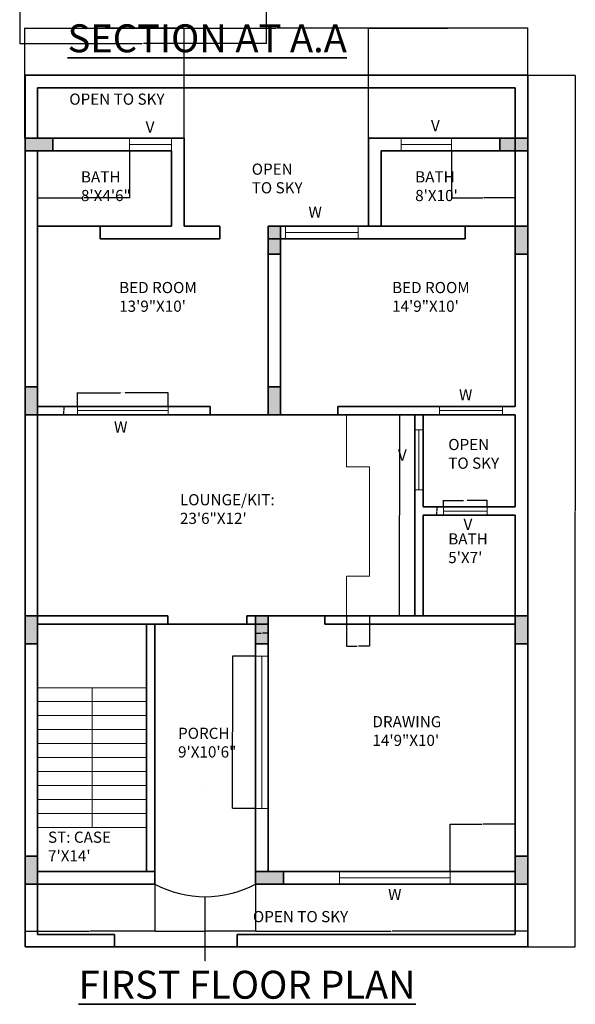
# Model space of a CAD drawing. Units: inches. Extents: x -29 to 834, y -635 to 572.
# Tile 2 of 4: x 434 to 832, y -635 to 69. Entities that reach past the tile are written whole.
import ezdxf

# ---------------------------------------------------------------- set-up
doc = ezdxf.new("R2010")
doc.units = ezdxf.units.IN
doc.header["$MEASUREMENT"] = 0
for name, color, linetype, lineweight in [('A-ANNO-DIMS', 2, 'Continuous', 18), ('A-ANNO-TITL', 7, 'Continuous', 35), ('A-AREA-IDEN', 7, 'Continuous', 18), ('A-COLS', 7, 'Continuous', 35), ('A-FLOR', 7, 'Continuous', 25), ('A-FLOR-FIXT', 8, 'Continuous', 18), ('A-FLOR-STRS', 3, 'Continuous', 18), ('A-GLAZ', 4, 'Continuous', 18), ('A-GLAZ-IDEN', 3, 'Continuous', 18), ('A-WALL', 7, 'Continuous', 35), ('C-PROP', 7, 'Continuous', 35)]:
    doc.layers.add(name, color=color, linetype=linetype, lineweight=lineweight)
doc.styles.get("Standard").update_dxf_attribs({"font": 'arial.ttf'})
doc.dimstyles.get("Standard").update_dxf_attribs({"dimtxt": 0.18, "dimasz": 0.18, "dimexe": 0.18, "dimexo": 0.0625, "dimgap": 0.09, "dimtad": 0, "dimtih": 1, "dimtoh": 1, "dimdec": 4, "dimzin": 0, "dimdsep": 46, "dimtxsty": 'Standard', "dimcen": 0.09, "dimadec": 0, "dimazin": 0, "dimtfac": 1, "dimtdec": 4, "dimtofl": 0, "dimtmove": 0, "dimatfit": 3, "dimfxl": 1, "dimtolj": 1, "dimtzin": 0, "dimarcsym": 0})

# ---------------------------------------------------------------- blocks, each defined once
blk = doc.blocks.new('STAIR-PLAN-RETURN-FLIGHT')
for p, q in [((78, 100), (0, 100)), ((39, 100), (39, 0)), ((78, 90), (0, 90)), ((78, 80), (0, 80)), ((78, 70), (0, 70)), ((78, 60), (0, 60)), ((78, 50), (0, 50)), ((78, 40), (0, 40)), ((78, 30), (0, 30)), ((78, 20), (0, 20)), ((78, 10), (0, 10)), ((78, 0), (0, 0))]:
    blk.add_line(p, q)
blk = doc.blocks.new('KITCHEN-COUNTER-PLAN')
for p, q in [((0, 144), (0, 106.7)), ((0, 106.7), (16.48, 106.7)), ((16.48, 106.7), (16.48, 28.5)), ((16.48, 28.5), (0, 28.5)), ((0, 28.5), (0, 0))]:
    blk.add_line(p, q)
blk = doc.blocks.new('WIN-DRAWING-FRONT-PLAN')
for p, q in [((0, 9), (0, 0)), ((79.05, 9), (79.05, 0)), ((79.05, 4.5), (0, 4.5))]:
    blk.add_line(p, q)
blk = doc.blocks.new('WIN-PORCH-SIDE-PLAN')
for p, q in [((9, 109.08), (0, 109.08)), ((4.5, 0), (4.5, 109.08)), ((9, 0), (0, 0))]:
    blk.add_line(p, q)
blk = doc.blocks.new('WIN-BEDROOM-LOUNGE-PLAN')
for p, q in [((0, 0), (0, 6)), ((64.98, 3), (0, 3)), ((64.98, 0), (64.98, 6))]:
    blk.add_line(p, q)
blk = doc.blocks.new('VENT-LIGHTWELL-SIDE-PLAN')
for p, q in [((6, 43.01), (0, 43.01)), ((3, 0), (3, 43.01)), ((6, 0), (0, 0))]:
    blk.add_line(p, q)
blk = doc.blocks.new('WIN-BEDROOM-REAR-PLAN')
for p, q in [((0, 9), (0, 0)), ((52.22, 9), (52.22, 0)), ((0, 4.5), (52.22, 4.5))]:
    blk.add_line(p, q)
blk = doc.blocks.new('VENT-BATH-LIGHTWELL-PLAN')
for p, q in [((0, 0), (0, 6)), ((31.44, 3), (0, 3)), ((31.44, 0), (31.44, 6))]:
    blk.add_line(p, q)
blk = doc.blocks.new('WIN-BEDROOM-LIGHTWELL-PLAN')
for p, q in [((0, 6), (0, 0)), ((0, 3), (45.04, 3)), ((45.04, 6), (45.04, 0))]:
    blk.add_line(p, q)
blk = doc.blocks.new('VENT-REAR-BATH-R-PLAN')
for p, q in [((0, 9), (0, 0)), ((35.81, 9), (35.81, 0)), ((0, 4.5), (35.81, 4.5))]:
    blk.add_line(p, q)
blk = doc.blocks.new('VENT-REAR-BATH-L-PLAN')
for p, q in [((0, 9), (0, 0)), ((30.05, 9), (30.05, 0)), ((0, 4.5), (30.05, 4.5))]:
    blk.add_line(p, q)
blk = doc.blocks.new('COLUMN-9X20-PLAN')
h = blk.add_hatch(color=256)
h.dxf.hatch_style = 1
h.paths.add_polyline_path([(9, 20), (0, 20), (0, 0), (9, 0)])
blk.add_lwpolyline([(0, 20), (9, 20), (9, 0), (0, 0)], close=True)
blk = doc.blocks.new('*D25')
at = {"layer": 'A-ANNO-DIMS', "color": 0, "lineweight": -2, "transparency": 16777216}
for p, q in [((684.21, -213.46), (705.92, -213.46)), ((705.74, -213.64), (705.74, -285.27)), ((705.74, -357.28), (705.74, -285.64)), ((684.21, -357.46), (705.92, -357.46))]:
    blk.add_line(p, q, dxfattribs=at)
at = {"layer": 'A-ANNO-DIMS', "color": 0, "transparency": 16777216}
for points in [[(705.71, -213.64), (705.77, -213.64), (705.74, -213.46)], [(705.71, -357.28), (705.77, -357.28), (705.74, -357.46)]]:
    blk.add_solid(points, dxfattribs=at)
at = {"layer": 'DEFPOINTS', "color": 0, "transparency": 16777216}
for p in [(684.14, -213.46), (705.74, -213.46), (684.14, -357.46)]:
    blk.add_point(p, dxfattribs=at)
at = {"layer": 'A-ANNO-DIMS', "color": 0, "transparency": 16777216, "insert": (705.74, -285.46), "char_height": 0.18, "attachment_point": 5}
blk.add_mtext('\\A1;COUNTER 144 TYP.', dxfattribs=at)
blk = doc.blocks.new('*D26')
at = {"layer": 'A-ANNO-DIMS', "color": 0, "lineweight": -2, "transparency": 16777216}
for p, q in [((667.66, -357.52), (667.66, -379.24)), ((684.14, -357.52), (684.14, -379.24)), ((667.84, -379.06), (675.38, -379.06)), ((683.96, -379.06), (676.42, -379.06))]:
    blk.add_line(p, q, dxfattribs=at)
at = {"layer": 'A-ANNO-DIMS', "color": 0, "transparency": 16777216}
for points in [[(667.84, -379.03), (667.84, -379.09), (667.66, -379.06)], [(683.96, -379.03), (683.96, -379.09), (684.14, -379.06)]]:
    blk.add_solid(points, dxfattribs=at)
at = {"layer": 'DEFPOINTS', "color": 0, "transparency": 16777216}
for p in [(667.66, -357.46), (684.14, -357.46), (684.14, -379.06)]:
    blk.add_point(p, dxfattribs=at)
at = {"layer": 'A-ANNO-DIMS', "color": 0, "transparency": 16777216, "insert": (675.9, -379.06), "char_height": 0.18, "attachment_point": 5}
blk.add_mtext('\\A1;16 TYP.', dxfattribs=at)
blk = doc.blocks.new('*D29')
at = {"layer": 'A-ANNO-DIMS', "color": 0, "lineweight": -2, "transparency": 16777216}
for p, q in [((602.5, -386.17), (586.02, -386.17)), ((586.2, -386.35), (586.2, -440.52)), ((586.2, -495.06), (586.2, -440.89)), ((602.5, -495.24), (586.02, -495.24))]:
    blk.add_line(p, q, dxfattribs=at)
at = {"layer": 'A-ANNO-DIMS', "color": 0, "transparency": 16777216}
for points in [[(586.17, -386.35), (586.23, -386.35), (586.2, -386.17)], [(586.17, -495.06), (586.23, -495.06), (586.2, -495.24)]]:
    blk.add_solid(points, dxfattribs=at)
at = {"layer": 'DEFPOINTS', "color": 0, "transparency": 16777216}
for p in [(602.56, -386.17), (586.2, -495.24), (602.56, -495.24)]:
    blk.add_point(p, dxfattribs=at)
at = {"layer": 'A-ANNO-DIMS', "color": 0, "transparency": 16777216, "insert": (586.2, -440.71), "char_height": 0.18, "attachment_point": 5}
blk.add_mtext('\\A1;PORCH WINDOW 109 TYP.', dxfattribs=at)
blk = doc.blocks.new('*D30')
at = {"layer": 'A-ANNO-DIMS', "color": 0, "lineweight": -2, "transparency": 16777216}
for p, q in [((602.56, -386.1), (602.56, -369.62)), ((602.74, -369.8), (606.6, -369.8)), ((611.38, -369.8), (607.52, -369.8)), ((611.56, -386.1), (611.56, -369.62))]:
    blk.add_line(p, q, dxfattribs=at)
at = {"layer": 'A-ANNO-DIMS', "color": 0, "transparency": 16777216}
for points in [[(602.74, -369.77), (602.74, -369.83), (602.56, -369.8)], [(611.38, -369.77), (611.38, -369.83), (611.56, -369.8)]]:
    blk.add_solid(points, dxfattribs=at)
at = {"layer": 'DEFPOINTS', "color": 0, "transparency": 16777216}
for p in [(602.56, -369.8), (602.56, -386.17), (611.56, -386.17)]:
    blk.add_point(p, dxfattribs=at)
at = {"layer": 'A-ANNO-DIMS', "color": 0, "transparency": 16777216, "insert": (607.06, -369.8), "char_height": 0.18, "attachment_point": 5}
blk.add_mtext('\\A1;9 TYP.', dxfattribs=at)
blk = doc.blocks.new('*D31')
at = {"layer": 'A-ANNO-DIMS', "color": 0, "lineweight": -2, "transparency": 16777216}
for p, q in [((475.12, -207.39), (475.12, -197.53)), ((475.3, -197.71), (505.93, -197.71)), ((539.92, -197.71), (509.29, -197.71)), ((540.1, -207.39), (540.1, -197.53))]:
    blk.add_line(p, q, dxfattribs=at)
at = {"layer": 'A-ANNO-DIMS', "color": 0, "transparency": 16777216}
for points in [[(475.3, -197.68), (475.3, -197.74), (475.12, -197.71)], [(539.92, -197.68), (539.92, -197.74), (540.1, -197.71)]]:
    blk.add_solid(points, dxfattribs=at)
at = {"layer": 'DEFPOINTS', "color": 0, "transparency": 16777216}
for p in [(475.12, -197.71), (475.12, -207.46), (540.1, -207.46)]:
    blk.add_point(p, dxfattribs=at)
at = {"layer": 'A-ANNO-DIMS', "color": 0, "transparency": 16777216, "insert": (507.61, -197.71), "char_height": 0.18, "attachment_point": 5}
blk.add_mtext('\\A1;LOUNGE WINDOW 65 TYP.', dxfattribs=at)
blk = doc.blocks.new('*D32')
at = {"layer": 'A-ANNO-DIMS', "color": 0, "lineweight": -2, "transparency": 16777216}
for p, q in [((475.06, -207.46), (465.2, -207.46)), ((465.38, -207.64), (465.38, -210.28)), ((465.38, -213.28), (465.38, -210.64)), ((475.06, -213.46), (465.2, -213.46))]:
    blk.add_line(p, q, dxfattribs=at)
at = {"layer": 'A-ANNO-DIMS', "color": 0, "transparency": 16777216}
for points in [[(465.35, -207.64), (465.41, -207.64), (465.38, -207.46)], [(465.35, -213.28), (465.41, -213.28), (465.38, -213.46)]]:
    blk.add_solid(points, dxfattribs=at)
at = {"layer": 'DEFPOINTS', "color": 0, "transparency": 16777216}
for p in [(475.12, -207.46), (465.38, -213.46), (475.12, -213.46)]:
    blk.add_point(p, dxfattribs=at)
at = {"layer": 'A-ANNO-DIMS', "color": 0, "transparency": 16777216, "insert": (465.38, -210.46), "char_height": 0.18, "attachment_point": 5}
blk.add_mtext('\\A1;6 TYP.', dxfattribs=at)
blk = doc.blocks.new('*D37')
at = {"layer": 'A-ANNO-DIMS', "color": 0, "lineweight": -2, "transparency": 16777216}
for p, q in [((737.12, -279.39), (737.12, -274.56)), ((737.3, -274.74), (751.58, -274.74)), ((768.38, -274.74), (754.1, -274.74)), ((768.56, -279.39), (768.56, -274.56))]:
    blk.add_line(p, q, dxfattribs=at)
at = {"layer": 'A-ANNO-DIMS', "color": 0, "transparency": 16777216}
for points in [[(737.3, -274.71), (737.3, -274.77), (737.12, -274.74)], [(768.38, -274.71), (768.38, -274.77), (768.56, -274.74)]]:
    blk.add_solid(points, dxfattribs=at)
at = {"layer": 'DEFPOINTS', "color": 0, "transparency": 16777216}
for p in [(737.12, -274.74), (737.12, -279.46), (768.56, -279.46)]:
    blk.add_point(p, dxfattribs=at)
at = {"layer": 'A-ANNO-DIMS', "color": 0, "transparency": 16777216, "insert": (752.84, -274.74), "char_height": 0.18, "attachment_point": 5}
blk.add_mtext('\\A1;BATH VENT 31 TYP.', dxfattribs=at)
blk = doc.blocks.new('*D38')
at = {"layer": 'A-ANNO-DIMS', "color": 0, "lineweight": -2, "transparency": 16777216}
for p, q in [((737.06, -279.46), (732.22, -279.46)), ((732.4, -279.64), (732.4, -282.28)), ((737.06, -285.46), (732.22, -285.46)), ((732.4, -285.28), (732.4, -282.64))]:
    blk.add_line(p, q, dxfattribs=at)
at = {"layer": 'A-ANNO-DIMS', "color": 0, "transparency": 16777216}
for points in [[(732.37, -279.64), (732.43, -279.64), (732.4, -279.46)], [(732.37, -285.28), (732.43, -285.28), (732.4, -285.46)]]:
    blk.add_solid(points, dxfattribs=at)
at = {"layer": 'DEFPOINTS', "color": 0, "transparency": 16777216}
for p in [(737.12, -279.46), (732.4, -285.46), (737.12, -285.46)]:
    blk.add_point(p, dxfattribs=at)
at = {"layer": 'A-ANNO-DIMS', "color": 0, "transparency": 16777216, "insert": (732.4, -282.46), "char_height": 0.18, "attachment_point": 5}
blk.add_mtext('\\A1;6 TYP.', dxfattribs=at)
blk = doc.blocks.new('*D61')
at = {"layer": 'A-ANNO-DIMS', "color": 0, "lineweight": -2, "transparency": 16777216}
for p, q in [((437.56, 29.61), (437.56, 63.52)), ((797.56, 29.61), (797.56, 63.52)), ((437.74, 63.34), (617.27, 63.34)), ((797.38, 63.34), (617.85, 63.34))]:
    blk.add_line(p, q, dxfattribs=at)
at = {"layer": 'A-ANNO-DIMS', "color": 0, "transparency": 16777216}
for points in [[(437.74, 63.37), (437.74, 63.31), (437.56, 63.34)], [(797.38, 63.37), (797.38, 63.31), (797.56, 63.34)]]:
    blk.add_solid(points, dxfattribs=at)
at = {"layer": 'DEFPOINTS', "color": 0, "transparency": 16777216}
for p in [(797.56, 63.34), (437.56, 29.54), (797.56, 29.54)]:
    blk.add_point(p, dxfattribs=at)
at = {"layer": 'A-ANNO-DIMS', "color": 0, "transparency": 16777216, "insert": (617.56, 63.34), "char_height": 0.18, "attachment_point": 5}
blk.add_mtext('\\A1;360', dxfattribs=at)
blk = doc.blocks.new('*D62')
at = {"layer": 'A-ANNO-DIMS', "color": 0, "lineweight": -2, "transparency": 16777216}
for p, q in [((797.63, 29.54), (831.54, 29.54)), ((831.36, 29.36), (831.36, -282.28)), ((831.36, -594.28), (831.36, -282.64)), ((797.63, -594.46), (831.54, -594.46))]:
    blk.add_line(p, q, dxfattribs=at)
at = {"layer": 'A-ANNO-DIMS', "color": 0, "transparency": 16777216}
for points in [[(831.33, 29.36), (831.39, 29.36), (831.36, 29.54)], [(831.33, -594.28), (831.39, -594.28), (831.36, -594.46)]]:
    blk.add_solid(points, dxfattribs=at)
at = {"layer": 'DEFPOINTS', "color": 0, "transparency": 16777216}
for p in [(797.56, 29.54), (831.36, 29.54), (797.56, -594.46)]:
    blk.add_point(p, dxfattribs=at)
at = {"layer": 'A-ANNO-DIMS', "color": 0, "transparency": 16777216, "insert": (831.36, -282.46), "char_height": 0.18, "attachment_point": 5}
blk.add_mtext('\\A1;624', dxfattribs=at)
blk = doc.blocks.new('*D63')
at = {"layer": 'A-ANNO-DIMS', "color": 0, "lineweight": -2, "transparency": 16777216}
for p, q in [((437.56, -549.52), (437.56, -583.44)), ((530.56, -549.52), (530.56, -583.44)), ((437.74, -583.26), (483.84, -583.26)), ((530.38, -583.26), (484.28, -583.26))]:
    blk.add_line(p, q, dxfattribs=at)
at = {"layer": 'A-ANNO-DIMS', "color": 0, "transparency": 16777216}
for points in [[(437.74, -583.23), (437.74, -583.29), (437.56, -583.26)], [(530.38, -583.23), (530.38, -583.29), (530.56, -583.26)]]:
    blk.add_solid(points, dxfattribs=at)
at = {"layer": 'DEFPOINTS', "color": 0, "transparency": 16777216}
for p in [(437.56, -549.46), (530.56, -549.46), (437.56, -583.26)]:
    blk.add_point(p, dxfattribs=at)
at = {"layer": 'A-ANNO-DIMS', "color": 0, "transparency": 16777216, "insert": (484.06, -583.26), "char_height": 0.18, "attachment_point": 5}
blk.add_mtext('\\A1;93', dxfattribs=at)
blk = doc.blocks.new('*D64')
at = {"layer": 'A-ANNO-DIMS', "color": 0, "lineweight": -2, "transparency": 16777216}
for p, q in [((530.56, -549.52), (530.56, -583.44)), ((602.56, -549.52), (602.56, -583.44)), ((530.74, -583.26), (566.35, -583.26)), ((602.38, -583.26), (566.78, -583.26))]:
    blk.add_line(p, q, dxfattribs=at)
at = {"layer": 'A-ANNO-DIMS', "color": 0, "transparency": 16777216}
for points in [[(530.74, -583.23), (530.74, -583.29), (530.56, -583.26)], [(602.38, -583.23), (602.38, -583.29), (602.56, -583.26)]]:
    blk.add_solid(points, dxfattribs=at)
at = {"layer": 'DEFPOINTS', "color": 0, "transparency": 16777216}
for p in [(530.56, -549.46), (602.56, -549.46), (530.56, -583.26)]:
    blk.add_point(p, dxfattribs=at)
at = {"layer": 'A-ANNO-DIMS', "color": 0, "transparency": 16777216, "insert": (566.56, -583.26), "char_height": 0.18, "attachment_point": 5}
blk.add_mtext('\\A1;72', dxfattribs=at)
blk = doc.blocks.new('*D65')
at = {"layer": 'A-ANNO-DIMS', "color": 0, "lineweight": -2, "transparency": 16777216}
for p, q in [((602.56, -549.52), (602.56, -583.44)), ((797.56, -549.52), (797.56, -583.44)), ((602.74, -583.26), (699.78, -583.26)), ((797.38, -583.26), (700.34, -583.26))]:
    blk.add_line(p, q, dxfattribs=at)
at = {"layer": 'A-ANNO-DIMS', "color": 0, "transparency": 16777216}
for points in [[(602.74, -583.23), (602.74, -583.29), (602.56, -583.26)], [(797.38, -583.23), (797.38, -583.29), (797.56, -583.26)]]:
    blk.add_solid(points, dxfattribs=at)
at = {"layer": 'DEFPOINTS', "color": 0, "transparency": 16777216}
for p in [(602.56, -549.46), (797.56, -549.46), (602.56, -583.26)]:
    blk.add_point(p, dxfattribs=at)
at = {"layer": 'A-ANNO-DIMS', "color": 0, "transparency": 16777216, "insert": (700.06, -583.26), "char_height": 0.18, "attachment_point": 5}
blk.add_mtext('\\A1;195', dxfattribs=at)
blk = doc.blocks.new('*D72')
at = {"layer": 'A-ANNO-DIMS', "color": 0, "lineweight": -2, "transparency": 16777216}
for p, q in [((437.56, -15.39), (437.56, 63.52)), ((551.56, -15.39), (551.56, 63.52)), ((437.74, 63.34), (494.28, 63.34)), ((551.38, 63.34), (494.84, 63.34))]:
    blk.add_line(p, q, dxfattribs=at)
at = {"layer": 'A-ANNO-DIMS', "color": 0, "transparency": 16777216}
for points in [[(437.74, 63.37), (437.74, 63.31), (437.56, 63.34)], [(551.38, 63.37), (551.38, 63.31), (551.56, 63.34)]]:
    blk.add_solid(points, dxfattribs=at)
at = {"layer": 'DEFPOINTS', "color": 0, "transparency": 16777216}
for p in [(551.56, 63.34), (437.56, -15.46), (551.56, -15.46)]:
    blk.add_point(p, dxfattribs=at)
at = {"layer": 'A-ANNO-DIMS', "color": 0, "transparency": 16777216, "insert": (494.56, 63.34), "char_height": 0.18, "attachment_point": 5}
blk.add_mtext('\\A1;114', dxfattribs=at)
blk = doc.blocks.new('*D73')
at = {"layer": 'A-ANNO-DIMS', "color": 0, "lineweight": -2, "transparency": 16777216}
for p, q in [((551.56, -15.39), (551.56, 63.52)), ((683.56, -15.39), (683.56, 63.52)), ((551.74, 63.34), (617.28, 63.34)), ((683.38, 63.34), (617.84, 63.34))]:
    blk.add_line(p, q, dxfattribs=at)
at = {"layer": 'A-ANNO-DIMS', "color": 0, "transparency": 16777216}
for points in [[(551.74, 63.37), (551.74, 63.31), (551.56, 63.34)], [(683.38, 63.37), (683.38, 63.31), (683.56, 63.34)]]:
    blk.add_solid(points, dxfattribs=at)
at = {"layer": 'DEFPOINTS', "color": 0, "transparency": 16777216}
for p in [(683.56, 63.34), (551.56, -15.46), (683.56, -15.46)]:
    blk.add_point(p, dxfattribs=at)
at = {"layer": 'A-ANNO-DIMS', "color": 0, "transparency": 16777216, "insert": (617.56, 63.34), "char_height": 0.18, "attachment_point": 5}
blk.add_mtext('\\A1;132', dxfattribs=at)
blk = doc.blocks.new('*D74')
at = {"layer": 'A-ANNO-DIMS', "color": 0, "lineweight": -2, "transparency": 16777216}
for p, q in [((683.56, -15.39), (683.56, 63.52)), ((797.56, -15.39), (797.56, 63.52)), ((683.74, 63.34), (740.28, 63.34)), ((797.38, 63.34), (740.84, 63.34))]:
    blk.add_line(p, q, dxfattribs=at)
at = {"layer": 'A-ANNO-DIMS', "color": 0, "transparency": 16777216}
for points in [[(683.74, 63.37), (683.74, 63.31), (683.56, 63.34)], [(797.38, 63.37), (797.38, 63.31), (797.56, 63.34)]]:
    blk.add_solid(points, dxfattribs=at)
at = {"layer": 'DEFPOINTS', "color": 0, "transparency": 16777216}
for p in [(797.56, 63.34), (683.56, -15.46), (797.56, -15.46)]:
    blk.add_point(p, dxfattribs=at)
at = {"layer": 'A-ANNO-DIMS', "color": 0, "transparency": 16777216, "insert": (740.56, 63.34), "char_height": 0.18, "attachment_point": 5}
blk.add_mtext('\\A1;114', dxfattribs=at)
blk = doc.blocks.new('*D75')
at = {"layer": 'A-ANNO-DIMS', "color": 0, "lineweight": -2, "transparency": 16777216}
for p, q in [((446.56, -24.52), (446.56, -58.44)), ((512.45, -24.52), (512.45, -58.44)), ((446.74, -58.26), (479.11, -58.26)), ((512.27, -58.26), (479.9, -58.26))]:
    blk.add_line(p, q, dxfattribs=at)
at = {"layer": 'A-ANNO-DIMS', "color": 0, "transparency": 16777216}
for points in [[(446.74, -58.23), (446.74, -58.29), (446.56, -58.26)], [(512.27, -58.23), (512.27, -58.29), (512.45, -58.26)]]:
    blk.add_solid(points, dxfattribs=at)
at = {"layer": 'DEFPOINTS', "color": 0, "transparency": 16777216}
for p in [(446.56, -24.46), (512.45, -24.46), (446.56, -58.26)]:
    blk.add_point(p, dxfattribs=at)
at = {"layer": 'A-ANNO-DIMS', "color": 0, "transparency": 16777216, "insert": (479.51, -58.26), "char_height": 0.18, "attachment_point": 5}
blk.add_mtext('\\A1;65.89', dxfattribs=at)
blk = doc.blocks.new('*D76')
at = {"layer": 'A-ANNO-DIMS', "color": 0, "lineweight": -2, "transparency": 16777216}
for p, q in [((742.81, -24.52), (742.81, -58.44)), ((788.56, -24.52), (788.56, -58.44)), ((742.99, -58.26), (765.29, -58.26)), ((788.38, -58.26), (766.08, -58.26))]:
    blk.add_line(p, q, dxfattribs=at)
at = {"layer": 'A-ANNO-DIMS', "color": 0, "transparency": 16777216}
for points in [[(742.99, -58.23), (742.99, -58.29), (742.81, -58.26)], [(788.38, -58.23), (788.38, -58.29), (788.56, -58.26)]]:
    blk.add_solid(points, dxfattribs=at)
at = {"layer": 'DEFPOINTS', "color": 0, "transparency": 16777216}
for p in [(742.81, -24.46), (788.56, -24.46), (742.81, -58.26)]:
    blk.add_point(p, dxfattribs=at)
at = {"layer": 'A-ANNO-DIMS', "color": 0, "transparency": 16777216, "insert": (765.68, -58.26), "char_height": 0.18, "attachment_point": 5}
blk.add_mtext('\\A1;45.76', dxfattribs=at)
blk = doc.blocks.new('*D79')
at = {"layer": 'A-ANNO-DIMS', "color": 0, "lineweight": -2, "transparency": 16777216}
for p, q in [((741.86, -540.39), (741.86, -506.48)), ((742.04, -506.66), (764.88, -506.66)), ((788.38, -506.66), (765.54, -506.66)), ((788.56, -540.39), (788.56, -506.48))]:
    blk.add_line(p, q, dxfattribs=at)
at = {"layer": 'A-ANNO-DIMS', "color": 0, "transparency": 16777216}
for points in [[(742.04, -506.63), (742.04, -506.69), (741.86, -506.66)], [(788.38, -506.63), (788.38, -506.69), (788.56, -506.66)]]:
    blk.add_solid(points, dxfattribs=at)
at = {"layer": 'DEFPOINTS', "color": 0, "transparency": 16777216}
for p in [(788.56, -506.66), (741.86, -540.46), (788.56, -540.46)]:
    blk.add_point(p, dxfattribs=at)
at = {"layer": 'A-ANNO-DIMS', "color": 0, "transparency": 16777216, "insert": (765.21, -506.66), "char_height": 0.18, "attachment_point": 5}
blk.add_mtext('\\A1;46.7', dxfattribs=at)
blk = doc.blocks.new('*D101')
at = {"layer": 'A-ANNO-DIMS', "color": 0, "lineweight": -2, "transparency": 16777216}
for p, q in [((433.76, 110.48), (433.76, 52.17)), ((610.21, 110.48), (610.21, 52.17)), ((433.94, 52.35), (521.53, 52.35)), ((610.03, 52.35), (522.44, 52.35))]:
    blk.add_line(p, q, dxfattribs=at)
at = {"layer": 'A-ANNO-DIMS', "color": 0, "transparency": 16777216}
for points in [[(433.94, 52.38), (433.94, 52.32), (433.76, 52.35)], [(610.03, 52.38), (610.03, 52.32), (610.21, 52.35)]]:
    blk.add_solid(points, dxfattribs=at)
at = {"layer": 'DEFPOINTS', "color": 0, "transparency": 16777216}
for p in [(433.76, 110.54), (610.21, 110.54), (610.21, 52.35)]:
    blk.add_point(p, dxfattribs=at)
at = {"layer": 'A-ANNO-DIMS', "color": 0, "transparency": 16777216, "insert": (521.98, 52.35), "char_height": 0.18, "attachment_point": 5}
blk.add_mtext('\\A1;176.45', dxfattribs=at)
blk = doc.blocks.new('*D108')
at = {"layer": 'A-ANNO-DIMS', "color": 0, "lineweight": -2, "transparency": 16777216}
for p, q in [((566.47, -481.96), (566.65, -481.96)), ((566.56, -482.05), (566.56, -481.87)), ((566.56, -604.36), (566.56, -558.64)), ((566.74, -604.36), (566.56, -604.36))]:
    blk.add_line(p, q, dxfattribs=at)
at = {"layer": 'A-ANNO-DIMS', "color": 0, "transparency": 16777216}
blk.add_solid([(566.59, -558.64), (566.53, -558.64), (566.56, -558.46)], dxfattribs=at)
at = {"layer": 'DEFPOINTS', "color": 0, "transparency": 16777216}
for p in [(566.56, -481.96), (566.56, -558.46)]:
    blk.add_point(p, dxfattribs=at)
at = {"layer": 'A-ANNO-DIMS', "color": 0, "transparency": 16777216, "insert": (567.15, -604.36), "char_height": 0.18, "attachment_point": 5}
blk.add_mtext('\\A1;R76.5', dxfattribs=at)

msp = doc.modelspace()

# ---------------------------------------------------------------- linework, layer by layer
at = {"layer": 'A-FLOR'}
msp.add_arc((566.5626, -481.957), 76.5, 241.9275073, 298.0724927, dxfattribs=at)
at = {"layer": 'A-WALL'}
for p, q in [((446.5626, 20.5431), (788.5626, 20.5431)), ((446.5626, 20.5431), (446.5626, -15.4569)), ((788.5626, 20.5431), (788.5626, -78.4569)), ((446.5626, -15.4569), (551.5626, -15.4569)), ((551.5626, -15.4569), (551.5626, -78.4569)), ((683.5626, -15.4569), (788.5626, -15.4569)), ((683.5626, -15.4569), (683.5626, -78.4569)), ((446.5626, -24.4569), (542.5626, -24.4569)), ((446.5626, -24.4569), (446.5626, -78.4569)), ((542.5626, -24.4569), (542.5626, -78.4569)), ((692.5626, -24.4569), (788.5626, -24.4569)), ((692.5626, -24.4569), (692.5626, -78.4569)), ((446.5626, -78.4569), (542.5626, -78.4569)), ((446.5626, -78.4569), (446.5626, -87.4569)), ((491.4048, -78.4569), (491.4048, -87.4569)), ((551.5626, -78.4569), (577.0558, -78.4569)), ((577.0558, -78.4569), (577.0558, -87.4569)), ((611.5626, -78.4569), (788.5626, -78.4569)), ((611.5626, -78.4569), (611.5626, -207.4569)), ((752.6848, -78.4569), (752.6848, -87.4569)), ((788.5626, -78.4569), (788.5626, -87.4569)), ((446.5626, -87.4569), (446.5626, -207.4569)), ((491.4048, -87.4569), (577.0558, -87.4569)), ((611.5626, -87.4569), (752.6848, -87.4569)), ((620.5626, -87.4569), (620.5626, -207.4569)), ((788.5626, -87.4569), (788.5626, -207.4569)), ((446.5626, -207.4569), (570.1065, -207.4569)), ((570.1065, -207.4569), (570.1065, -213.4569)), ((611.5626, -207.4569), (611.5626, -213.4569)), ((620.5626, -207.4569), (620.5626, -213.4569)), ((661.5051, -207.4569), (788.5626, -207.4569)), ((661.5051, -207.4569), (661.5051, -213.4569)), ((446.5626, -213.4569), (788.5626, -213.4569)), ((446.5626, -213.4569), (446.5626, -357.4569)), ((716.5626, -213.4569), (716.5626, -357.4569)), ((722.5626, -213.4569), (722.5626, -279.4569)), ((788.5626, -213.4569), (788.5626, -279.4569)), ((722.5626, -279.4569), (788.5626, -279.4569)), ((722.5626, -285.4569), (788.5626, -285.4569)), ((722.5626, -285.4569), (722.5626, -357.4569)), ((788.5626, -285.4569), (788.5626, -357.4569)), ((446.5626, -357.4569), (539.8795, -357.4569)), ((539.8795, -357.4569), (539.8795, -363.4569)), ((596.4793, -357.4569), (788.5626, -357.4569)), ((596.4793, -357.4569), (596.4793, -363.4569)), ((611.5626, -363.4569), (611.5626, -357.4569)), ((652.1881, -357.4569), (652.1881, -363.4569)), ((446.5626, -363.4569), (611.5626, -363.4569)), ((446.5626, -363.4569), (446.5626, -540.4569)), ((524.5626, -363.4569), (524.5626, -540.4569)), ((530.5626, -363.4569), (530.5626, -549.4569)), ((602.5626, -363.4569), (602.5626, -549.4569)), ((611.5626, -363.4569), (611.5626, -540.4569)), ((652.1881, -363.4569), (788.5626, -363.4569)), ((788.5626, -363.4569), (788.5626, -540.4569)), ((446.5626, -540.4569), (530.5626, -540.4569)), ((602.5626, -540.4569), (788.5626, -540.4569)), ((446.5626, -549.4569), (530.5626, -549.4569)), ((446.5626, -549.4569), (446.5626, -585.4569)), ((602.5626, -549.4569), (788.5626, -549.4569)), ((788.5626, -549.4569), (788.5626, -585.4569)), ((446.5626, -585.4569), (501.5833, -585.4569)), ((501.5833, -585.4569), (501.5833, -594.4569)), ((589.5168, -585.4569), (788.5626, -585.4569)), ((589.5168, -585.4569), (589.5168, -594.4569))]:
    msp.add_line(p, q, dxfattribs=at)
at = {"layer": 'C-PROP'}
for p, q in [((437.5626, 29.5431), (797.5626, 29.5431)), ((437.5626, 29.5431), (437.5626, -594.4569)), ((797.5626, 29.5431), (797.5626, -594.4569)), ((437.5626, -594.4569), (797.5626, -594.4569))]:
    msp.add_line(p, q, dxfattribs=at)

# ---------------------------------------------------------------- block references
at = {"layer": 'A-COLS'}
for p, rotation in [((437.5626, -15.4569), 270.0000000000002), ((777.5626, -15.4569), 270.0000000000002), ((602.5626, -540.4569), 269.9999999999995)]:
    msp.add_blockref('COLUMN-9X20-PLAN', p, dxfattribs=dict(at, rotation=rotation))
for p in [(611.5626, -98.4569), (788.5626, -98.4569), (437.5626, -213.4569), (611.5626, -213.4569), (437.5626, -377.4569), (602.5626, -377.4569), (788.5626, -377.4569), (437.5626, -549.4569), (788.5626, -549.4569)]:
    msp.add_blockref('COLUMN-9X20-PLAN', p, dxfattribs=at)
at = {"layer": 'A-FLOR-FIXT'}
msp.add_blockref('KITCHEN-COUNTER-PLAN', (667.661, -357.4569), dxfattribs=at)
at = {"layer": 'A-FLOR-STRS'}
msp.add_blockref('STAIR-PLAN-RETURN-FLIGHT', (446.5626, -508.8447), dxfattribs=at)
at = {"layer": 'A-GLAZ'}
for name, p in [('VENT-REAR-BATH-L-PLAN', (512.45, -24.4569)), ('VENT-REAR-BATH-R-PLAN', (707.0002, -24.4569)), ('WIN-BEDROOM-REAR-PLAN', (623.9837, -87.4569)), ('WIN-BEDROOM-LIGHTWELL-PLAN', (734.3077, -213.4569)), ('WIN-DRAWING-FRONT-PLAN', (662.8149, -549.4569))]:
    msp.add_blockref(name, p, dxfattribs=at)
at = {"layer": 'A-GLAZ', "rotation": 180}
for name, p in [('WIN-BEDROOM-LOUNGE-PLAN', (540.0997, -207.4569)), ('VENT-LIGHTWELL-SIDE-PLAN', (722.5626, -224.1814)), ('VENT-BATH-LIGHTWELL-PLAN', (768.5589, -279.4569)), ('WIN-PORCH-SIDE-PLAN', (611.5626, -386.1664))]:
    msp.add_blockref(name, p, dxfattribs=at)

# ---------------------------------------------------------------- texts
at = {"layer": 'A-ANNO-TITL', "char_height": 20, "attachment_point": 1}
for s, insert in [('{\\LSECTION AT A.A}', (468.0427, 66.0256)), ('{\\LFIRST FLOOR PLAN}', (475.9632, -611.4996))]:
    msp.add_mtext_dynamic_manual_height_columns(s, width=384.972308, gutter_width=1, heights=[0], dxfattribs=dict(at, insert=insert))
at = {"layer": 'A-AREA-IDEN', "char_height": 8, "attachment_point": 1}
for s, insert in [('OPEN TO SKY', (469.2703, 16.4692)), ('OPEN\\PTO SKY', (599.8903, -33.6457)), ('BATH\\P8\'X4\'6"', (477.6207, -39.1901)), ("BATH\\P8'X10'", (716.9232, -39.1901)), ('BED ROOM\\P13\'9"X10\'', (504.9938, -118.4186)), ('BED ROOM\\P14\'9"X10\'', (700.4035, -118.4186)), ('OPEN\\PTO SKY', (740.5888, -230.7819)), ('LOUNGE/KIT:\\P23\'6"X12\'', (548.5087, -270.2979)), ("BATH\\P5'X7'", (740.5888, -298.3415)), ('DRAWING\\P14\'9"X10\'', (686.3234, -429.2086)), ('PORCH\\P9\'X10\'6"', (547.1385, -437.4896)), ("ST: CASE\\P7'X14'", (454.0475, -511.8774)), ('OPEN TO SKY', (600.7441, -568.7152))]:
    msp.add_mtext_dynamic_manual_height_columns(s, width=92.580232, gutter_width=1, heights=[0], dxfattribs=dict(at, insert=insert))
at = {"layer": 'A-GLAZ-IDEN', "char_height": 8, "attachment_point": 1}
for s, width, insert in [('V', 15.530915, (523.9493, -3.4402)), ('V', 15.530915, (728.2293, -2.5018)), ('W', 92.580232, (640.5145, -64.4301)), ('W', 92.580232, (748.29, -195.1503)), ('W', 92.580232, (501.3218, -218.2872)), ('V', 15.530915, (704.5498, -238.3243)), ('V', 15.530915, (751.5533, -287.9574)), ('W', 92.580232, (697.5275, -552.8615))]:
    msp.add_mtext_dynamic_manual_height_columns(s, width=width, gutter_width=1, heights=[0], dxfattribs=dict(at, insert=insert))

# ---------------------------------------------------------------- dimensions: what is measured, and where the dimension line sits
at = {"layer": 'A-ANNO-DIMS'}
for base, p1, p2, override, picture, middle in [((610.2079, 52.3492), (433.7594, 110.5416), (610.2079, 110.5416), {"dimdec": 2, "dimlfac": 1, "dimrnd": 0, "dimzin": 0, "dimdsep": 46, "dimlunit": 2}, '*D101', (521.9837, 52.3492)), ((797.5626, 63.3431), (437.5626, 29.5431), (797.5626, 29.5431), {"dimdec": 0, "dimlfac": 1, "dimrnd": 0, "dimzin": 0, "dimdsep": 46, "dimlunit": 2}, '*D61', (617.5626, 63.3431)), ((551.5626, 63.3431), (437.5626, -15.4569), (551.5626, -15.4569), {"dimdec": 0, "dimlfac": 1, "dimrnd": 0, "dimzin": 0, "dimdsep": 46, "dimlunit": 2}, '*D72', (494.5626, 63.3431)), ((683.5626, 63.3431), (551.5626, -15.4569), (683.5626, -15.4569), {"dimdec": 0, "dimlfac": 1, "dimrnd": 0, "dimzin": 0, "dimdsep": 46, "dimlunit": 2}, '*D73', (617.5626, 63.3431)), ((797.5626, 63.3431), (683.5626, -15.4569), (797.5626, -15.4569), {"dimdec": 0, "dimlfac": 1, "dimrnd": 0, "dimzin": 0, "dimdsep": 46, "dimlunit": 2}, '*D74', (740.5626, 63.3431))]:
    dim = msp.add_linear_dim(base=base, p1=p1, p2=p2, dimstyle='Standard', override=override, dxfattribs=at)
    dim.commit()
    dim.dimension.update_dxf_attribs({"geometry": picture, "text_midpoint": middle})
for base, p1, p2, angle, override, picture, middle in [((831.3626, 29.5431), (797.5626, -594.4569), (797.5626, 29.5431), 90, {"dimdec": 0, "dimlfac": 1, "dimrnd": 0, "dimzin": 0, "dimdsep": 46, "dimlunit": 2}, '*D62', (831.3626, -282.4569)), ((446.5626, -58.2569), (512.45, -24.4569), (446.5626, -24.4569), 180, {"dimdec": 2, "dimlfac": 1, "dimrnd": 0, "dimzin": 0, "dimdsep": 46, "dimlunit": 2}, '*D75', (479.5063, -58.2569)), ((742.8066, -58.2569), (788.5626, -24.4569), (742.8066, -24.4569), 180, {"dimdec": 2, "dimlfac": 1, "dimrnd": 0, "dimzin": 0, "dimdsep": 46, "dimlunit": 2}, '*D76', (765.6846, -58.2569)), ((788.5626, -506.6569), (741.8605, -540.4569), (788.5626, -540.4569), 0, {"dimdec": 1, "dimlfac": 1, "dimrnd": 0, "dimzin": 0, "dimdsep": 46, "dimlunit": 2}, '*D79', (765.2115, -506.6569)), ((437.5626, -583.2569), (530.5626, -549.4569), (437.5626, -549.4569), 180, {"dimdec": 0, "dimlfac": 1, "dimrnd": 0, "dimzin": 0, "dimdsep": 46, "dimlunit": 2}, '*D63', (484.0626, -583.2569)), ((530.5626, -583.2569), (602.5626, -549.4569), (530.5626, -549.4569), 180, {"dimdec": 0, "dimlfac": 1, "dimrnd": 0, "dimzin": 0, "dimdsep": 46, "dimlunit": 2}, '*D64', (566.5626, -583.2569)), ((602.5626, -583.2569), (797.5626, -549.4569), (602.5626, -549.4569), 180, {"dimdec": 0, "dimlfac": 1, "dimrnd": 0, "dimzin": 0, "dimdsep": 46, "dimlunit": 2}, '*D65', (700.0626, -583.2569))]:
    dim = msp.add_linear_dim(base=base, p1=p1, p2=p2, angle=angle, dimstyle='Standard', override=override, dxfattribs=at)
    dim.commit()
    dim.dimension.update_dxf_attribs({"geometry": picture, "text_midpoint": middle})
for base, p1, p2, angle, text, picture, middle in [((475.1233, -197.7105), (540.0997, -207.4569), (475.1233, -207.4569), 180, 'LOUNGE WINDOW <> TYP.', '*D31', (507.6115, -197.7105)), ((465.3768, -213.4569), (475.1233, -207.4569), (475.1233, -213.4569), 270, '<> TYP.', '*D32', (465.3768, -210.4569)), ((705.7437, -213.4569), (684.1437, -357.4569), (684.1437, -213.4569), 90, 'COUNTER <> TYP.', '*D25', (705.7437, -285.4569)), ((737.1205, -274.7412), (768.5589, -279.4569), (737.1205, -279.4569), 180, 'BATH VENT <> TYP.', '*D37', (752.8397, -274.7412)), ((732.4048, -285.4569), (737.1205, -279.4569), (737.1205, -285.4569), 270, '<> TYP.', '*D38', (732.4048, -282.4569)), ((602.5626, -369.8047), (611.5626, -386.1664), (602.5626, -386.1664), 180, '<> TYP.', '*D30', (607.0626, -369.8047)), ((586.2009, -495.2445), (602.5626, -386.1664), (602.5626, -495.2445), 270, 'PORCH WINDOW <> TYP.', '*D29', (586.2009, -440.7054))]:
    dim = msp.add_linear_dim(base=base, p1=p1, p2=p2, angle=angle, text=text, dimstyle='Standard', override={"dimdec": 0, "dimlfac": 1, "dimrnd": 0, "dimzin": 0, "dimdsep": 46, "dimlunit": 2}, dxfattribs=at)
    dim.commit()
    dim.dimension.update_dxf_attribs({"geometry": picture, "text_midpoint": middle})
dim = msp.add_linear_dim(base=(684.1437, -379.0569), p1=(667.661, -357.4569), p2=(684.1437, -357.4569), text='<> TYP.', dimstyle='Standard', override={"dimdec": 0, "dimlfac": 1, "dimrnd": 0, "dimzin": 0, "dimdsep": 46, "dimlunit": 2}, dxfattribs=at)
dim.commit()
dim.dimension.update_dxf_attribs({"geometry": '*D26', "text_midpoint": (675.9023, -379.0569)})
dim = msp.add_radius_dim(center=(566.5626, -481.957), mpoint=(566.563, -558.4569), dimstyle='Standard', override={"dimdec": 1, "dimlfac": 1, "dimrnd": 0, "dimzin": 0, "dimdsep": 46, "dimlunit": 2}, dxfattribs=at)
dim.commit()
dim.dimension.update_dxf_attribs({"geometry": '*D108', "text_midpoint": (567.1538, -604.3569), "dimtype": 164})

doc.saveas('drawing.dxf')
